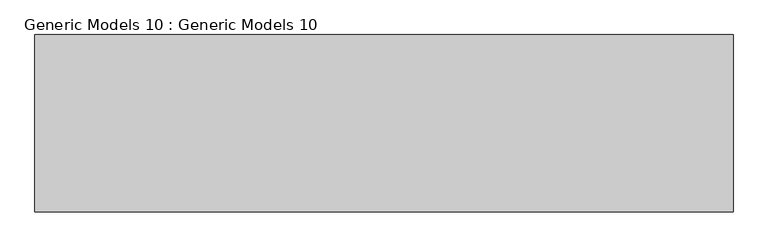
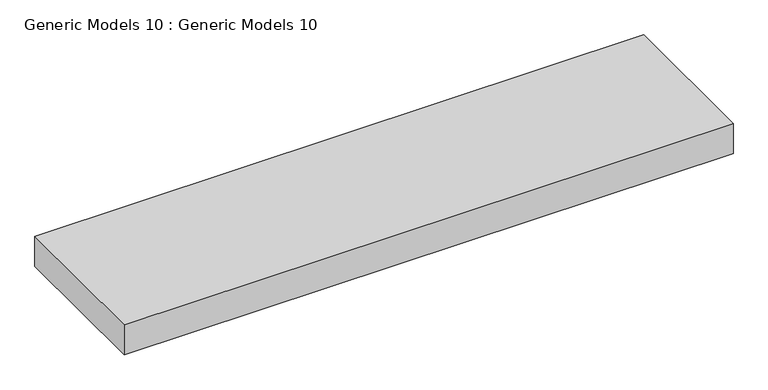
"""IFC4 building model written with IfcOpenShell, lengths in millimetres: proxy geometry, Generic Models 10 : Generic Models 10."""

from ifc_helpers import new_model, si_unit, frame, origin, place, context, project, spatial, polyline, outline, extrude, source, transform, mapped, element, save


def generic_models_10_generic_models_10_d4c633cf(model_context):
    return source(origin(), model_context, "Body", "SweptSolid", [
        extrude(outline(polyline([(-15576.2546109, 3583.9054373), (-15576.2546109, 4690.9207268), (-11218.1120831, 4690.9207268), (-11218.1120831, 3583.9054373), (-15576.2546109, 3583.9054373)])), frame((0.0, 0.0, 5462.9315541), z_axis=(0.0, 0.0, 1.0), x_axis=(1.0, 0.0, 0.0)), (0.0, 0.0, 1.0), 228.6),
    ])


if __name__ == "__main__":
    model = new_model("IFC4")
    model_context = context("Model", 3, world=origin())
    ifc_project = project(units=[si_unit("LENGTHUNIT", "METRE", prefix="MILLI")], contexts=[model_context])
    site = spatial("IfcSite", under=ifc_project)
    building = spatial("IfcBuilding", under=site)
    placement = place(None, origin())
    generic_models_10_generic_models_10_shape = generic_models_10_generic_models_10_d4c633cf(model_context)
    element("IfcBuildingElementProxy", 1, Name="Generic Models 10 : Generic Models 10", ObjectType="Generic Models 10 : Generic Models 10", at=placement, inside=building, context=model_context, shape_type="MappedRepresentation", body=[
        mapped(generic_models_10_generic_models_10_shape, transform((0.0, 0.0, 0.0), x_axis=(1.0, 0.0, 0.0), y_axis=(0.0, 1.0, 0.0), z_axis=(0.0, 0.0, 1.0))),
    ])
    save(model, "model.ifc")
